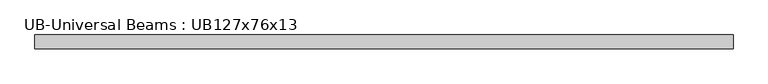
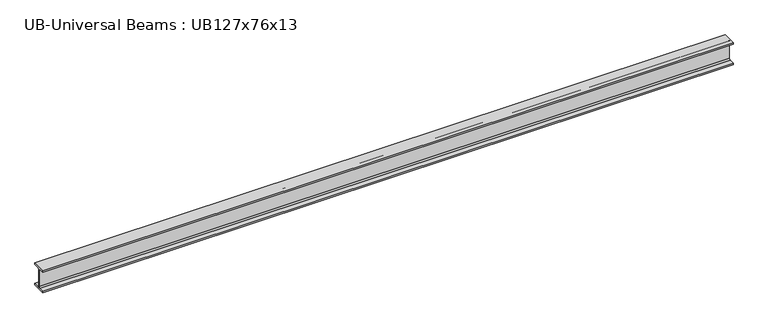
"""IFC4 building model written with IfcOpenShell, lengths in millimetres: member geometry, UB-Universal Beams : UB127x76x13."""

from ifc_helpers import new_model, si_unit, point, frame, frame_2d, origin, place, context, project, spatial, polyline, circle_curve, trimmed, segment, composite_curve, outline, extrude, source, transform, mapped, element, save


def ub_universal_beams_ub127x76x13_5289bed7(model_context):
    return source(origin(), model_context, "Body", "SweptSolid", [
        extrude(outline(composite_curve([segment(polyline([(38.0, -55.9), (38.0, -63.5), (-38.0, -63.5), (-38.0, -55.9), (-9.6, -55.9)]), True, "CONTINUOUS"), segment(trimmed(circle_curve(frame_2d((-9.6, -48.3)), 7.6), [point((-9.6, -55.9))], [point((-2.0, -48.3))], True, "CARTESIAN"), True, "CONTINUOUS"), segment(polyline([(-2.0, -48.3), (-2.0, 48.3)]), True, "CONTINUOUS"), segment(trimmed(circle_curve(frame_2d((-9.6, 48.3)), 7.6), [point((-2.0, 48.3))], [point((-9.6, 55.9))], True, "CARTESIAN"), True, "CONTINUOUS"), segment(polyline([(-9.6, 55.9), (-38.0, 55.9), (-38.0, 63.5), (38.0, 63.5), (38.0, 55.9), (9.6, 55.9)]), True, "CONTINUOUS"), segment(trimmed(circle_curve(frame_2d((9.6, 48.3)), 7.6), [point((9.6, 55.9))], [point((2.0, 48.3))], True, "CARTESIAN"), True, "CONTINUOUS"), segment(polyline([(2.0, 48.3), (2.0, -48.3)]), True, "CONTINUOUS"), segment(trimmed(circle_curve(frame_2d((9.6, -48.3)), 7.6), [point((2.0, -48.3))], [point((9.6, -55.9))], True, "CARTESIAN"), True, "CONTINUOUS"), segment(polyline([(9.6, -55.9), (38.0, -55.9)]), True, "CONTINUOUS")], self_intersect=False)), frame((-2124.8, 0.0, 0.0), z_axis=(1.0, 0.0, 0.0), x_axis=(0.0, 1.0, 0.0)), (0.0, 0.0, 1.0), 3810.4),
    ])


if __name__ == "__main__":
    model = new_model("IFC4")
    model_context = context("Model", 3, world=origin())
    ifc_project = project(units=[si_unit("LENGTHUNIT", "METRE", prefix="MILLI")], contexts=[model_context])
    site = spatial("IfcSite", under=ifc_project)
    building = spatial("IfcBuilding", under=site)
    placement = place(None, origin())
    ub_universal_beams_ub127x76x13_shape = ub_universal_beams_ub127x76x13_5289bed7(model_context)
    element("IfcMember", 1, ObjectType="UB-Universal Beams : UB127x76x13", at=placement, inside=building, context=model_context, shape_type="MappedRepresentation", body=[
        mapped(ub_universal_beams_ub127x76x13_shape, transform((0.0, 0.0, 0.0), x_axis=(1.0, 0.0, 0.0), y_axis=(0.0, 1.0, 0.0), z_axis=(0.0, 0.0, 1.0))),
    ])
    save(model, "model.ifc")

# Revit data of these elements
# Type "UB-Universal Beams : UB127x76x13"
#   Section Name Key = "UB127X76X13"
#   Width = 7.6 cm
#   Web Thickness = 0.4 cm
#   Web Fillet = 0.76 cm
#   Warping Constant = 2000.0 cm⁶
#   Torsional Moment of Inertia = 2.85 cm⁴
#   Section Area = 16.5 cm²
#   Plastic Modulus weak axis = 22.6 cm³
#   Plastic Modulus strong axis = 84.2 cm³
#   Nominal Weight = 13.00 kgf/m
#   Moment of Inertia weak axis = 55.70 cm⁴
#   Moment of Inertia strong axis = 473.00 cm⁴
#   Height = 12.7 cm
#   Flange Thickness = 0.76 cm
#   Elastic Modulus weak axis = 14.7 cm³
#   Elastic Modulus strong axis = 74.6 cm³
#   Centroid Vertical = 6.35 cm
#   Centroid Horizontal = 3.8 cm
#   Bolt Spacing = 4.0 cm
#   Length [instance default] = 1.5 m
#   Structural Material [instance default] = Metal - Steel 43-275
#   Type Comments = ""
#   Assembly Code = ""
# Element 1 (IfcMember, "UB-Universal Beams : UB127x76x13")
#   Materials on its faces: "Metal - Steel 43-275"
# Materials
#   "Metal - Steel 43-275": class "Metal", colour RGB 247 247 247, transparency 0, Cost = 0
